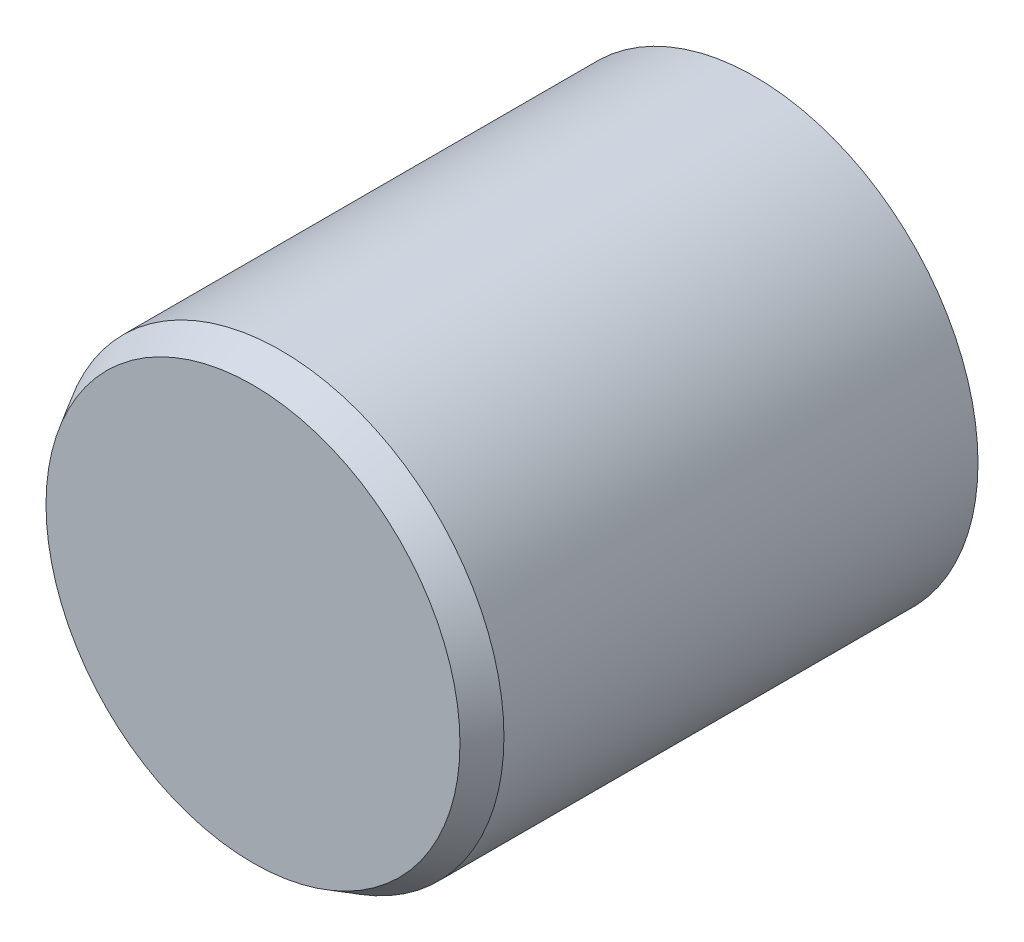
SolidWorks part; units mm, degrees
material "Plain Carbon Steel"
ref_plane "Front Plane" through (0, 0, 0) normal (0, 0, 1) x (1, 0, 0)
ref_plane "Top Plane" through (0, 0, 0) normal (0, 1, 0) x (1, 0, 0)
ref_plane "Right Plane" through (0, 0, 0) normal (1, 0, 0) x (0, 0, -1)
sketch "Pin Profile Sketch" plane through (0, 0, 0) normal (1, 0, 0) x (0, 0, -1)
  line L0 (0, -1.4667) -> (0, -2.9667)
  line L1 (0, -2.9667) -> (-9, -2.9667)
  line L2 (-9, -2.9667) -> (-9, 1.0333)
  line L3 (-9, 1.0333) -> (-6, 1.0333)
  line L4 (-6, 1.0333) -> (-6, -1.4667)
  line L5 (-6, -1.4667) -> (0, -1.4667)
  line L6 (0, 2.96) -> (0, -1.4667) construction
  dimension "D1" = 9
  dimension "D2" = 6
  dimension "D3" = 2.5
  dimension "D4" = 4
  dimension "D5" = 1.0333
revolve "Pin Body Revolve" add sketch "Pin Profile Sketch" angle 360 about L3
chamfer "End Chamfer 0.5x30deg" distance 0.5 angle 30 1 edges at (4, 1.0333, 9)
